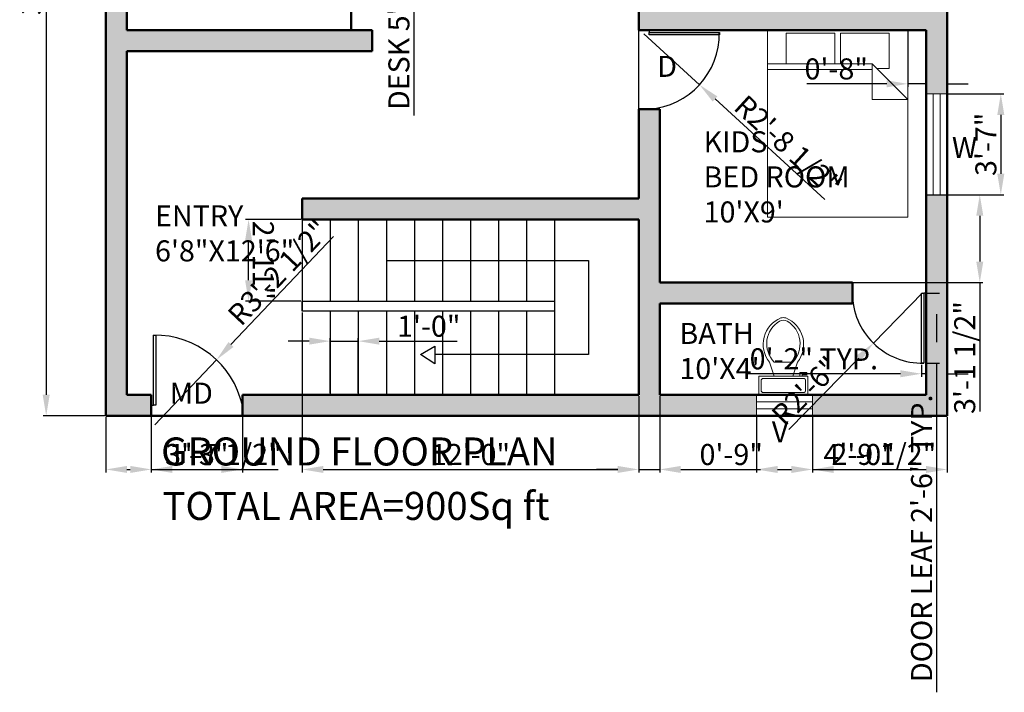
# Model space of a CAD drawing. Units: inches. Extents: x 16989 to 17950, y 7982 to 8536.
# Tile 1 of 5: x 16993 to 17415, y 7982 to 8270. Entities that reach past the tile are written whole.
import ezdxf

# ---------------------------------------------------------------- set-up
doc = ezdxf.new("R2010")
doc.units = ezdxf.units.IN
for name, color, linetype, lineweight in [('A-ANNO-DIMS', 2, 'Continuous', 18), ('A-ANNO-IDEN', 7, 'Continuous', 18), ('A-ANNO-TEXT', 7, 'Continuous', 35), ('A-AREA-IDEN', 7, 'Continuous', 25), ('A-DOOR', 3, 'Continuous', 25), ('A-FLOR-FIXT', 9, 'Continuous', 18), ('A-FLOR-STRS', 7, 'Continuous', 25), ('A-FURN', 8, 'Continuous', 18), ('A-GLAZ', 4, 'Continuous', 18), ('A-WALL', 7, 'Continuous', 50)]:
    doc.layers.add(name, color=color, linetype=linetype, lineweight=lineweight)
doc.layers.add('A-WALL-PATT', color=177, linetype='Continuous', lineweight=13, true_color=0x293189)
doc.styles.get("Standard").update_dxf_attribs({"font": 'arial.ttf'})
doc.dimstyles.new('ISO-25', dxfattribs={"dimtxt": 9, "dimasz": 9, "dimexe": 1.25, "dimexo": 0.625, "dimtad": 1, "dimdec": 1, "dimrnd": 9, "dimlunit": 3, "dimtxsty": 'Standard', "dimcen": 2.5, "dimadec": 0, "dimazin": 0, "dimtfac": 1, "dimtdec": 1, "dimtmove": 0, "dimatfit": 3, "dimfxl": 1, "dimarcsym": 0})

# ---------------------------------------------------------------- blocks, each defined once
blk = doc.blocks.new('Bed - Queen')
for p, q in [((0, -80.00003), (0, 0)), ((0, 0), (59.99999, 0)), ((59.99999, 0), (59.99999, -80.00003)), ((7.99999, -1.2), (28.79998, -1.2)), ((7.99999, -14.4), (7.99999, -1.2)), ((28.79998, -1.2), (28.79998, -14.4)), ((31.19999, -1.2), (51.99999, -1.2)), ((31.19999, -14.4), (31.19999, -1.2)), ((51.99999, -1.2), (51.99999, -16.4)), ((0, -14.4), (44.8, -14.4)), ((44.8, -16.8), (0, -16.8)), ((59.99999, -29.6), (44.8, -14.4)), ((44.8, -14.4), (44.8, -29.6)), ((51.99999, -16.4), (46.79936, -16.4)), ((44.8, -29.6), (59.99999, -29.6)), ((59.99999, -80.00003), (0, -80.00003))]:
    blk.add_line(p, q)
blk = doc.blocks.new('Toilet - top')
for p, q in [((9.5, -6), (9.5, -2)), ((-8, -8.5), (-8, -8)), ((-7, -8), (-7, -9.5)), ((-4, -8), (-6, -14)), ((4, -8), (6, -14)), ((-10, -8.5), (-8, -8.5)), ((-10, -9.5), (-10, -8.5)), ((-7, -9.5), (-10, -9.5)), ((4, -14), (-4, -14))]:
    blk.add_line(p, q)
blk.add_lwpolyline([(10.5, -8), (10.5, 0), (-10.5, 0), (-10.5, -8)], close=True)
for points in [[(-9.5, -2), (-9.5, -6)], [(8.5, -1), (-8.5, -1)], [(-8.5, -7), (8.5, -7)]]:
    blk.add_lwpolyline(points)
for centre, radius, start, end in [((-8.62, -1.88), 0.884, 81.8699, 188.1301), ((8.62, -1.88), 0.884, 351.8699, 98.1301), ((-8.62, -6.12), 0.884, 171.8699, 278.1301), ((8.62, -6.12), 0.884, 261.8699, 8.1301), ((3.52, -21.58), 12.17, 141.4691, 247.9714), ((4.2, -21.82), 11.33, 136.3677, 238.9468), ((-3.52, -21.58), 12.17, 292.0284, 38.5307), ((-4.2, -21.82), 11.33, 301.053, 43.6321), ((0, -27.88), 4, 245.7318, 294.2682), ((0, -29), 4, 254.8605, 285.1395)]:
    blk.add_arc(centre, radius, start, end)
blk = doc.blocks.new('*D9')
at = {"layer": 'A-ANNO-DIMS', "color": 0, "lineweight": -2, "transparency": 16777216}
for p, q in [((17029.59, 8460.26), (17003.42, 8460.26)), ((17004.67, 8451.26), (17004.67, 8109.26)), ((17029.59, 8100.26), (17003.42, 8100.26))]:
    blk.add_line(p, q, dxfattribs=at)
at = {"layer": 'A-ANNO-DIMS', "color": 0, "transparency": 16777216}
for points in [[(17003.17, 8451.26), (17006.17, 8451.26), (17004.67, 8460.26)], [(17003.17, 8109.26), (17006.17, 8109.26), (17004.67, 8100.26)]]:
    blk.add_solid(points, dxfattribs=at)
at = {"layer": 'Defpoints', "color": 0, "transparency": 16777216}
for p in [(17030.22, 8460.26), (17004.67, 8100.26), (17030.22, 8100.26)]:
    blk.add_point(p, dxfattribs=at)
at = {"layer": 'A-ANNO-DIMS', "color": 0, "transparency": 16777216, "insert": (16999.45, 8280.26), "char_height": 9, "attachment_point": 5, "rotation": 90}
blk.add_mtext("30'", dxfattribs=at)
blk = doc.blocks.new('DOOR-LEAF-30IN')
for p, q in [((1, 0), (1, 30)), ((1, 30), (2, 30)), ((2, 30), (2, 0)), ((0, 0), (1, 0)), ((2, 0), (1, 0))]:
    blk.add_line(p, q)
blk = doc.blocks.new('*D17')
at = {"layer": 'A-ANNO-DIMS', "color": 0, "lineweight": -2, "transparency": 16777216}
for p, q in [((17381.84, 8152.76), (17386.97, 8152.76)), ((17385.72, 8143.76), (17385.72, 8131.76)), ((17381.84, 8122.76), (17386.97, 8122.76)), ((17385.72, 8122.76), (17385.72, 7981.95))]:
    blk.add_line(p, q, dxfattribs=at)
at = {"layer": 'A-ANNO-DIMS', "color": 0, "transparency": 16777216}
for points in [[(17384.22, 8143.76), (17387.22, 8143.76), (17385.72, 8152.76)], [(17384.22, 8131.76), (17387.22, 8131.76), (17385.72, 8122.76)]]:
    blk.add_solid(points, dxfattribs=at)
at = {"layer": 'Defpoints', "color": 0, "transparency": 16777216}
for p in [(17381.22, 8152.76), (17381.22, 8122.76), (17385.72, 8122.76)]:
    blk.add_point(p, dxfattribs=at)
at = {"layer": 'A-ANNO-DIMS', "color": 0, "transparency": 16777216, "insert": (17380.44, 8047.85), "char_height": 9, "attachment_point": 5, "rotation": 90}
blk.add_mtext('DOOR LEAF 2\'-6" TYP.', dxfattribs=at)
blk = doc.blocks.new('*D18')
at = {"layer": 'A-ANNO-DIMS', "color": 0, "lineweight": -2, "transparency": 16777216}
for p, q in [((17379.22, 8122.14), (17379.22, 8117.01)), ((17381.22, 8122.14), (17381.22, 8117.01)), ((17370.22, 8118.26), (17305.11, 8118.26)), ((17381.22, 8118.26), (17379.22, 8118.26)), ((17390.22, 8118.26), (17399.22, 8118.26))]:
    blk.add_line(p, q, dxfattribs=at)
at = {"layer": 'A-ANNO-DIMS', "color": 0, "transparency": 16777216}
for points in [[(17370.22, 8119.76), (17370.22, 8116.76), (17379.22, 8118.26)], [(17390.22, 8119.76), (17390.22, 8116.76), (17381.22, 8118.26)]]:
    blk.add_solid(points, dxfattribs=at)
at = {"layer": 'Defpoints', "color": 0, "transparency": 16777216}
for p in [(17379.22, 8122.76), (17381.22, 8122.76), (17379.22, 8118.26)]:
    blk.add_point(p, dxfattribs=at)
at = {"layer": 'A-ANNO-DIMS', "color": 0, "transparency": 16777216, "insert": (17333.16, 8123.48), "char_height": 9, "attachment_point": 5}
blk.add_mtext('0\'-2" TYP.', dxfattribs=at)
blk = doc.blocks.new('*D27')
at = {"layer": 'A-ANNO-DIMS', "color": 0, "lineweight": -2, "transparency": 16777216}
for p, q in [((17170.41, 8391.11), (17160.79, 8391.11)), ((17162.04, 8382.11), (17162.04, 8340.11)), ((17170.41, 8331.11), (17160.79, 8331.11)), ((17162.04, 8331.11), (17162.04, 8228.71))]:
    blk.add_line(p, q, dxfattribs=at)
at = {"layer": 'A-ANNO-DIMS', "color": 0, "transparency": 16777216}
for points in [[(17160.54, 8382.11), (17163.54, 8382.11), (17162.04, 8391.11)], [(17160.54, 8340.11), (17163.54, 8340.11), (17162.04, 8331.11)]]:
    blk.add_solid(points, dxfattribs=at)
at = {"layer": 'Defpoints', "color": 0, "transparency": 16777216}
for p in [(17171.04, 8391.11), (17162.04, 8331.11), (17171.04, 8331.11)]:
    blk.add_point(p, dxfattribs=at)
at = {"layer": 'A-ANNO-DIMS', "color": 0, "transparency": 16777216, "insert": (17156.76, 8275.41), "char_height": 9, "attachment_point": 5, "rotation": 90}
blk.add_mtext('DESK 5\'-0" TYP.', dxfattribs=at)
blk = doc.blocks.new('*D33')
at = {"layer": 'A-ANNO-DIMS', "color": 0, "lineweight": -2, "transparency": 16777216}
for p, q in [((17042.78, 8293.82), (17042.78, 8279.54)), ((17133.78, 8293.82), (17133.78, 8279.54)), ((17051.78, 8280.79), (17124.78, 8280.79)), ((17133.78, 8280.79), (17242.95, 8280.79))]:
    blk.add_line(p, q, dxfattribs=at)
at = {"layer": 'A-ANNO-DIMS', "color": 0, "transparency": 16777216}
for points in [[(17051.78, 8282.29), (17051.78, 8279.29), (17042.78, 8280.79)], [(17124.78, 8282.29), (17124.78, 8279.29), (17133.78, 8280.79)]]:
    blk.add_solid(points, dxfattribs=at)
at = {"layer": 'Defpoints', "color": 0, "transparency": 16777216}
for p in [(17042.78, 8294.44), (17133.78, 8294.44), (17133.78, 8280.79)]:
    blk.add_point(p, dxfattribs=at)
at = {"layer": 'A-ANNO-DIMS', "color": 0, "transparency": 16777216, "insert": (17192.87, 8286.07), "char_height": 9, "attachment_point": 5}
blk.add_mtext('DINING SET 7\'-7"', dxfattribs=at)
blk = doc.blocks.new('*D43')
at = {"layer": 'A-ANNO-DIMS', "color": 0, "lineweight": -2, "transparency": 16777216}
for p, q in [((17381.84, 8194.87), (17405.42, 8194.87)), ((17404.17, 8185.87), (17404.17, 8166.26)), ((17381.84, 8157.26), (17405.42, 8157.26)), ((17404.17, 8157.26), (17404.17, 8102.12))]:
    blk.add_line(p, q, dxfattribs=at)
at = {"layer": 'A-ANNO-DIMS', "color": 0, "transparency": 16777216}
for points in [[(17402.67, 8185.87), (17405.67, 8185.87), (17404.17, 8194.87)], [(17402.67, 8166.26), (17405.67, 8166.26), (17404.17, 8157.26)]]:
    blk.add_solid(points, dxfattribs=at)
at = {"layer": 'Defpoints', "color": 0, "transparency": 16777216}
for p in [(17381.22, 8194.87), (17381.22, 8157.26), (17404.17, 8157.26)]:
    blk.add_point(p, dxfattribs=at)
at = {"layer": 'A-ANNO-DIMS', "color": 0, "transparency": 16777216, "insert": (17398.89, 8125.19), "char_height": 9, "attachment_point": 5, "rotation": 90}
blk.add_mtext('3\'-1 1/2"', dxfattribs=at)
blk = doc.blocks.new('*D44')
at = {"layer": 'A-ANNO-DIMS', "color": 0, "lineweight": -2, "transparency": 16777216}
for p, q in [((17390.84, 8238), (17414.42, 8238)), ((17413.17, 8229), (17413.17, 8203.87)), ((17390.84, 8194.87), (17414.42, 8194.87))]:
    blk.add_line(p, q, dxfattribs=at)
at = {"layer": 'A-ANNO-DIMS', "color": 0, "transparency": 16777216}
for points in [[(17411.67, 8229), (17414.67, 8229), (17413.17, 8238)], [(17411.67, 8203.87), (17414.67, 8203.87), (17413.17, 8194.87)]]:
    blk.add_solid(points, dxfattribs=at)
at = {"layer": 'Defpoints', "color": 0, "transparency": 16777216}
for p in [(17390.22, 8238), (17390.22, 8194.87), (17413.17, 8194.87)]:
    blk.add_point(p, dxfattribs=at)
at = {"layer": 'A-ANNO-DIMS', "color": 0, "transparency": 16777216, "insert": (17407.95, 8216.44), "char_height": 9, "attachment_point": 5, "rotation": 90}
blk.add_mtext('3\'-7"', dxfattribs=at)
blk = doc.blocks.new('*D47')
at = {"layer": 'A-ANNO-DIMS', "color": 0, "lineweight": -2, "transparency": 16777216}
for p, q in [((17030.22, 8099.64), (17030.22, 8076.06)), ((17049.62, 8099.64), (17049.62, 8076.06)), ((17039.22, 8077.31), (17040.62, 8077.31)), ((17049.62, 8077.31), (17103.92, 8077.31))]:
    blk.add_line(p, q, dxfattribs=at)
at = {"layer": 'A-ANNO-DIMS', "color": 0, "transparency": 16777216}
for points in [[(17039.22, 8078.81), (17039.22, 8075.81), (17030.22, 8077.31)], [(17040.62, 8078.81), (17040.62, 8075.81), (17049.62, 8077.31)]]:
    blk.add_solid(points, dxfattribs=at)
at = {"layer": 'Defpoints', "color": 0, "transparency": 16777216}
for p in [(17030.22, 8100.26), (17049.62, 8100.26), (17049.62, 8077.31)]:
    blk.add_point(p, dxfattribs=at)
at = {"layer": 'A-ANNO-DIMS', "color": 0, "transparency": 16777216, "insert": (17081.27, 8082.59), "char_height": 9, "attachment_point": 5}
blk.add_mtext('1\'-7 1/2"', dxfattribs=at)
blk = doc.blocks.new('*D48')
at = {"layer": 'A-ANNO-DIMS', "color": 0, "lineweight": -2, "transparency": 16777216}
for p, q in [((17049.62, 8099.64), (17049.62, 8076.06)), ((17088.6, 8099.64), (17088.6, 8076.06)), ((17058.62, 8077.31), (17079.6, 8077.31))]:
    blk.add_line(p, q, dxfattribs=at)
at = {"layer": 'A-ANNO-DIMS', "color": 0, "transparency": 16777216}
for points in [[(17058.62, 8078.81), (17058.62, 8075.81), (17049.62, 8077.31)], [(17079.6, 8078.81), (17079.6, 8075.81), (17088.6, 8077.31)]]:
    blk.add_solid(points, dxfattribs=at)
at = {"layer": 'Defpoints', "color": 0, "transparency": 16777216}
for p in [(17049.62, 8100.26), (17088.6, 8100.26), (17088.6, 8077.31)]:
    blk.add_point(p, dxfattribs=at)
at = {"layer": 'A-ANNO-DIMS', "color": 0, "transparency": 16777216, "insert": (17069.11, 8082.53), "char_height": 9, "attachment_point": 5}
blk.add_mtext('3\'-3"', dxfattribs=at)
blk = doc.blocks.new('*D49')
at = {"layer": 'A-ANNO-DIMS', "color": 0, "lineweight": -2, "transparency": 16777216}
for p, q in [((17308.63, 8099.64), (17308.63, 8076.06)), ((17332.58, 8099.64), (17332.58, 8076.06)), ((17317.63, 8077.31), (17323.58, 8077.31)), ((17332.58, 8077.31), (17366.91, 8077.31))]:
    blk.add_line(p, q, dxfattribs=at)
at = {"layer": 'A-ANNO-DIMS', "color": 0, "transparency": 16777216}
for points in [[(17317.63, 8078.81), (17317.63, 8075.81), (17308.63, 8077.31)], [(17323.58, 8078.81), (17323.58, 8075.81), (17332.58, 8077.31)]]:
    blk.add_solid(points, dxfattribs=at)
at = {"layer": 'Defpoints', "color": 0, "transparency": 16777216}
for p in [(17308.63, 8100.26), (17332.58, 8100.26), (17332.58, 8077.31)]:
    blk.add_point(p, dxfattribs=at)
at = {"layer": 'A-ANNO-DIMS', "color": 0, "transparency": 16777216, "insert": (17354.25, 8082.53), "char_height": 9, "attachment_point": 5}
blk.add_mtext('2\'-0"', dxfattribs=at)
blk = doc.blocks.new('*D50')
at = {"layer": 'A-ANNO-DIMS', "color": 0, "lineweight": -2, "transparency": 16777216}
for p, q in [((17332.58, 8099.64), (17332.58, 8076.06)), ((17390.22, 8099.64), (17390.22, 8076.06)), ((17341.58, 8077.31), (17381.22, 8077.31))]:
    blk.add_line(p, q, dxfattribs=at)
at = {"layer": 'A-ANNO-DIMS', "color": 0, "transparency": 16777216}
for points in [[(17341.58, 8078.81), (17341.58, 8075.81), (17332.58, 8077.31)], [(17381.22, 8078.81), (17381.22, 8075.81), (17390.22, 8077.31)]]:
    blk.add_solid(points, dxfattribs=at)
at = {"layer": 'Defpoints', "color": 0, "transparency": 16777216}
for p in [(17332.58, 8100.26), (17390.22, 8100.26), (17390.22, 8077.31)]:
    blk.add_point(p, dxfattribs=at)
at = {"layer": 'A-ANNO-DIMS', "color": 0, "transparency": 16777216, "insert": (17361.4, 8082.59), "char_height": 9, "attachment_point": 5}
blk.add_mtext('4\'-9 1/2"', dxfattribs=at)
blk = doc.blocks.new('*D61')
at = {"layer": 'A-ANNO-DIMS', "color": 0, "lineweight": -2, "transparency": 16777216}
for p, q in [((17114.22, 8144.4), (17114.22, 8076.06)), ((17258.22, 8108.64), (17258.22, 8076.06)), ((17123.22, 8077.31), (17249.22, 8077.31))]:
    blk.add_line(p, q, dxfattribs=at)
at = {"layer": 'A-ANNO-DIMS', "color": 0, "transparency": 16777216}
for points in [[(17123.22, 8078.81), (17123.22, 8075.81), (17114.22, 8077.31)], [(17249.22, 8078.81), (17249.22, 8075.81), (17258.22, 8077.31)]]:
    blk.add_solid(points, dxfattribs=at)
at = {"layer": 'Defpoints', "color": 0, "transparency": 16777216}
for p in [(17114.22, 8145.02), (17258.22, 8109.26), (17258.22, 8077.31)]:
    blk.add_point(p, dxfattribs=at)
at = {"layer": 'A-ANNO-DIMS', "color": 0, "transparency": 16777216, "insert": (17186.22, 8082.53), "char_height": 9, "attachment_point": 5}
blk.add_mtext('12\'-0"', dxfattribs=at)
blk = doc.blocks.new('*D62')
at = {"layer": 'A-ANNO-DIMS', "color": 0, "lineweight": -2, "transparency": 16777216}
for p, q in [((17113.59, 8184.26), (17090.01, 8184.25)), ((17091.27, 8158.3), (17091.26, 8175.25)), ((17113.59, 8149.31), (17090.02, 8149.3))]:
    blk.add_line(p, q, dxfattribs=at)
at = {"layer": 'A-ANNO-DIMS', "color": 0, "transparency": 16777216}
for points in [[(17092.76, 8175.26), (17089.76, 8175.25), (17091.26, 8184.25)], [(17092.77, 8158.3), (17089.77, 8158.3), (17091.27, 8149.3)]]:
    blk.add_solid(points, dxfattribs=at)
at = {"layer": 'Defpoints', "color": 0, "transparency": 16777216}
for p in [(17091.26, 8184.25), (17114.21, 8184.26), (17114.22, 8149.31)]:
    blk.add_point(p, dxfattribs=at)
at = {"layer": 'A-ANNO-DIMS', "color": 0, "transparency": 16777216, "insert": (17096.41, 8166.78), "char_height": 9, "attachment_point": 5, "rotation": 270.0146}
blk.add_mtext('2\'-11"', dxfattribs=at)
blk = doc.blocks.new('*D63')
at = {"layer": 'A-ANNO-DIMS', "color": 0, "lineweight": -2, "transparency": 16777216}
for p, q in [((17117.22, 8132.21), (17108.22, 8132.21)), ((17126.22, 8109.89), (17126.22, 8133.46)), ((17126.22, 8132.21), (17138.22, 8132.21)), ((17138.22, 8109.89), (17138.22, 8133.46)), ((17147.22, 8132.21), (17180.55, 8132.21))]:
    blk.add_line(p, q, dxfattribs=at)
at = {"layer": 'A-ANNO-DIMS', "color": 0, "transparency": 16777216}
for points in [[(17117.22, 8133.71), (17117.22, 8130.71), (17126.22, 8132.21)], [(17147.22, 8133.71), (17147.22, 8130.71), (17138.22, 8132.21)]]:
    blk.add_solid(points, dxfattribs=at)
at = {"layer": 'Defpoints', "color": 0, "transparency": 16777216}
for p in [(17138.22, 8132.21), (17126.22, 8109.26), (17138.22, 8109.26)]:
    blk.add_point(p, dxfattribs=at)
at = {"layer": 'A-ANNO-DIMS', "color": 0, "transparency": 16777216, "insert": (17168.38, 8137.43), "char_height": 9, "attachment_point": 5}
blk.add_mtext('1\'-0"', dxfattribs=at)
blk = doc.blocks.new('*D67')
at = {"layer": 'A-ANNO-DIMS', "color": 0, "lineweight": -2, "transparency": 16777216}
for p, q in [((17258.22, 8108.64), (17258.22, 8076.06)), ((17267.22, 8108.64), (17267.22, 8076.06)), ((17249.22, 8077.31), (17240.22, 8077.31)), ((17258.22, 8077.31), (17267.22, 8077.31)), ((17276.22, 8077.31), (17310.39, 8077.31))]:
    blk.add_line(p, q, dxfattribs=at)
at = {"layer": 'A-ANNO-DIMS', "color": 0, "transparency": 16777216}
for points in [[(17249.22, 8078.81), (17249.22, 8075.81), (17258.22, 8077.31)], [(17276.22, 8078.81), (17276.22, 8075.81), (17267.22, 8077.31)]]:
    blk.add_solid(points, dxfattribs=at)
at = {"layer": 'Defpoints', "color": 0, "transparency": 16777216}
for p in [(17258.22, 8109.26), (17267.22, 8109.26), (17267.22, 8077.31)]:
    blk.add_point(p, dxfattribs=at)
at = {"layer": 'A-ANNO-DIMS', "color": 0, "transparency": 16777216, "insert": (17297.81, 8082.53), "char_height": 9, "attachment_point": 5}
blk.add_mtext('0\'-9"', dxfattribs=at)
blk = doc.blocks.new('*D69')
at = {"layer": 'A-ANNO-DIMS', "color": 0, "lineweight": -2, "transparency": 16777216}
for p, q in [((17373.35, 8264.64), (17373.35, 8241.06)), ((17381.22, 8264.64), (17381.22, 8241.06)), ((17364.35, 8242.31), (17330.18, 8242.31)), ((17381.22, 8242.31), (17373.35, 8242.31)), ((17390.22, 8242.31), (17399.22, 8242.31))]:
    blk.add_line(p, q, dxfattribs=at)
at = {"layer": 'A-ANNO-DIMS', "color": 0, "transparency": 16777216}
for points in [[(17364.35, 8243.81), (17364.35, 8240.81), (17373.35, 8242.31)], [(17390.22, 8243.81), (17390.22, 8240.81), (17381.22, 8242.31)]]:
    blk.add_solid(points, dxfattribs=at)
at = {"layer": 'Defpoints', "color": 0, "transparency": 16777216}
for p in [(17373.35, 8265.26), (17381.22, 8265.26), (17373.35, 8242.31)]:
    blk.add_point(p, dxfattribs=at)
at = {"layer": 'A-ANNO-DIMS', "color": 0, "transparency": 16777216, "insert": (17342.76, 8247.53), "char_height": 9, "attachment_point": 5}
blk.add_mtext('0\'-8"', dxfattribs=at)
blk = doc.blocks.new('*D72')
at = {"layer": 'A-ANNO-DIMS', "color": 0, "lineweight": -2, "transparency": 16777216}
for p, q in [((17260.37, 8263.76), (17284.23, 8241.92)), ((17337.9, 8192.78), (17290.87, 8235.84))]:
    blk.add_line(p, q, dxfattribs=at)
at = {"layer": 'A-ANNO-DIMS', "color": 0, "transparency": 16777216}
blk.add_solid([(17291.88, 8236.94), (17289.86, 8234.73), (17284.23, 8241.92)], dxfattribs=at)
at = {"layer": 'Defpoints', "color": 0, "transparency": 16777216}
for p in [(17260.37, 8263.76), (17284.23, 8241.92)]:
    blk.add_point(p, dxfattribs=at)
at = {"layer": 'A-ANNO-DIMS', "color": 0, "transparency": 16777216, "insert": (17321.27, 8215.16), "char_height": 9, "attachment_point": 5, "rotation": 317.522}
blk.add_mtext('R2\'-8 1/2"', dxfattribs=at)
blk = doc.blocks.new('*D74')
at = {"layer": 'A-ANNO-DIMS', "color": 0, "lineweight": -2, "transparency": 16777216}
for p, q in [((17379.72, 8152.84), (17358.65, 8131.36)), ((17322.39, 8094.39), (17352.35, 8124.94))]:
    blk.add_line(p, q, dxfattribs=at)
at = {"layer": 'A-ANNO-DIMS', "color": 0, "transparency": 16777216}
blk.add_solid([(17351.28, 8125.99), (17353.42, 8123.89), (17358.65, 8131.36)], dxfattribs=at)
at = {"layer": 'Defpoints', "color": 0, "transparency": 16777216}
for p in [(17379.72, 8152.84), (17358.65, 8131.36)]:
    blk.add_point(p, dxfattribs=at)
at = {"layer": 'A-ANNO-DIMS', "color": 0, "transparency": 16777216, "insert": (17330.49, 8110.11), "char_height": 9, "attachment_point": 5, "rotation": 45.552}
blk.add_mtext('R2\'-6"', dxfattribs=at)
blk = doc.blocks.new('*D76')
at = {"layer": 'A-ANNO-DIMS', "color": 0, "lineweight": -2, "transparency": 16777216}
for p, q in [((17127.6, 8177.04), (17083.74, 8130.76)), ((17051.12, 8096.36), (17077.55, 8124.23))]:
    blk.add_line(p, q, dxfattribs=at)
at = {"layer": 'A-ANNO-DIMS', "color": 0, "transparency": 16777216}
blk.add_solid([(17082.65, 8131.8), (17084.83, 8129.73), (17077.55, 8124.23)], dxfattribs=at)
at = {"layer": 'Defpoints', "color": 0, "transparency": 16777216}
for p in [(17077.55, 8124.23), (17051.12, 8096.36)]:
    blk.add_point(p, dxfattribs=at)
at = {"layer": 'A-ANNO-DIMS', "color": 0, "transparency": 16777216, "insert": (17104.93, 8160.8), "char_height": 9, "attachment_point": 5, "rotation": 46.5334}
blk.add_mtext('R3\'-2 1/2"', dxfattribs=at)

msp = doc.modelspace()

# ---------------------------------------------------------------- hatches: boundary and pattern name
at = {"layer": 'A-WALL-PATT'}
h = msp.add_hatch(color=256, dxfattribs=at)
h.dxf.hatch_style = 1
h.paths.add_polyline_path([(17039.22, 8310.16), (17030.22, 8310.16), (17030.22, 8100.26), (17049.62, 8100.26), (17049.62, 8109.26), (17039.22, 8109.26), (17039.22, 8256.26), (17144.22, 8256.26), (17144.22, 8265.26), (17039.22, 8265.26)])
h.paths.add_polyline_path([(17039.22, 8451.26), (17065.89, 8451.26), (17065.89, 8460.26), (17030.22, 8460.26), (17030.22, 8357.88), (17039.22, 8357.88)])
h.paths.add_polyline_path([(17180.39, 8460.26), (17105.01, 8460.26), (17105.01, 8451.26), (17135.22, 8451.26), (17135.22, 8333.76), (17144.22, 8333.76), (17144.22, 8451.26), (17180.39, 8451.26)])
h.paths.add_polyline_path([(17309.67, 8460.26), (17217.66, 8460.26), (17217.66, 8451.26), (17258.22, 8451.26), (17258.22, 8304.98), (17262.72, 8304.98, -0.013209), (17264.26, 8304.98), (17267.22, 8304.98), (17267.22, 8394.26), (17348.26, 8394.26), (17348.26, 8403.26), (17267.22, 8403.26), (17267.22, 8451.26), (17309.67, 8451.26)])
h.paths.add_polyline_path([(17390.22, 8460.26), (17336.17, 8460.26), (17336.17, 8451.26), (17381.22, 8451.26), (17381.22, 8403.26), (17381.22, 8394.26), (17381.22, 8367.17), (17390.22, 8367.17)])
h.paths.add_polyline_path([(17390.22, 8325.05), (17381.22, 8325.05), (17381.22, 8274.26), (17267.22, 8274.26), (17258.22, 8274.26), (17258.22, 8265.26), (17267.22, 8265.26), (17381.22, 8265.26), (17381.22, 8238), (17390.22, 8238)])
h.paths.add_polyline_path([(17390.22, 8194.87), (17381.22, 8194.87), (17381.22, 8157.26), (17381.22, 8148.26), (17381.22, 8109.26), (17332.58, 8109.26), (17332.58, 8100.26), (17390.22, 8100.26)])
h.paths.add_polyline_path([(17349.64, 8157.26), (17267.22, 8157.26), (17267.22, 8231.5), (17258.22, 8231.5), (17258.22, 8193.26), (17144.22, 8193.26), (17114.21, 8193.26), (17114.21, 8184.26), (17144.22, 8184.26), (17258.22, 8184.26), (17258.22, 8109.26), (17088.6, 8109.26), (17088.6, 8100.26), (17308.63, 8100.26), (17308.63, 8109.26), (17267.22, 8109.26), (17267.22, 8148.26), (17349.64, 8148.26)])

# ---------------------------------------------------------------- linework, layer by layer
at = {"layer": 'A-DOOR'}
for p, q in [((17258.22, 8231.5), (17258.22, 8265.26)), ((17349.64, 8157.26), (17381.22, 8157.26))]:
    msp.add_line(p, q, dxfattribs=at)
for centre, radius, start, end in [((17260.37, 8263.76), 32.35, 274.1572, 0.8856), ((17379.72, 8152.84), 30.08, 180.1517, 270.9523), ((17051.12, 8096.36), 38.41, 12.64, 90.7459)]:
    msp.add_arc(centre, radius, start, end, dxfattribs=at)
at = {"layer": 'A-FLOR-STRS'}
for p, q in [((17114.22, 8184.26), (17114.22, 8145.02)), ((17126.22, 8184.26), (17126.22, 8149.31)), ((17138.22, 8184.26), (17138.22, 8149.31)), ((17150.22, 8184.26), (17150.22, 8149.31)), ((17162.22, 8184.26), (17162.22, 8149.31)), ((17174.22, 8184.26), (17174.22, 8149.31)), ((17186.22, 8184.26), (17186.22, 8149.31)), ((17198.22, 8184.26), (17198.22, 8149.31)), ((17210.22, 8184.26), (17210.22, 8149.31)), ((17222.22, 8184.26), (17222.22, 8109.26)), ((17150.22, 8166.79), (17236.68, 8166.79)), ((17236.68, 8166.79), (17236.68, 8126.43)), ((17126.22, 8145.02), (17126.22, 8109.26)), ((17138.22, 8145.02), (17138.22, 8109.26)), ((17150.22, 8145.02), (17150.22, 8109.26)), ((17162.22, 8145.02), (17162.22, 8109.26)), ((17174.22, 8145.02), (17174.22, 8109.26)), ((17186.22, 8145.02), (17186.22, 8109.26)), ((17198.22, 8145.02), (17198.22, 8109.26)), ((17210.22, 8145.02), (17210.22, 8109.26)), ((17164.87, 8126.43), (17171.03, 8130.06)), ((17171.03, 8130.06), (17171.03, 8122.45)), ((17171.03, 8122.45), (17164.87, 8126.43)), ((17236.68, 8126.43), (17171.03, 8126.43))]:
    msp.add_line(p, q, dxfattribs=at)
msp.add_lwpolyline([(17222.22, 8145.02), (17114.22, 8145.02), (17114.22, 8149.31), (17222.22, 8149.31)], close=True, dxfattribs=at)
at = {"layer": 'A-GLAZ'}
for p, q in [((17381.22, 8238), (17390.22, 8238)), ((17384.22, 8194.87), (17384.22, 8238)), ((17387.22, 8194.87), (17387.22, 8238)), ((17381.22, 8194.87), (17390.22, 8194.87)), ((17308.63, 8109.26), (17308.63, 8100.26)), ((17332.58, 8109.26), (17332.58, 8100.26)), ((17308.63, 8106.26), (17332.58, 8106.26)), ((17308.63, 8103.26), (17332.58, 8103.26))]:
    msp.add_line(p, q, dxfattribs=at)
at = {"layer": 'A-WALL'}
for p, q in [((17030.22, 8460.26), (17030.22, 8100.26)), ((17390.22, 8100.26), (17390.22, 8460.26)), ((17039.22, 8451.26), (17039.22, 8265.26)), ((17135.22, 8451.26), (17135.22, 8265.26)), ((17258.22, 8274.26), (17258.22, 8265.26)), ((17144.22, 8265.26), (17039.22, 8265.26)), ((17144.22, 8265.26), (17144.22, 8256.26)), ((17267.22, 8265.26), (17258.22, 8265.26)), ((17381.22, 8265.26), (17267.22, 8265.26)), ((17381.22, 8157.26), (17381.22, 8265.26)), ((17144.22, 8256.26), (17039.22, 8256.26)), ((17039.22, 8256.26), (17039.22, 8109.26)), ((17267.22, 8231.5), (17258.22, 8231.5)), ((17258.22, 8231.5), (17258.22, 8193.26)), ((17267.22, 8231.5), (17267.22, 8157.26)), ((17144.22, 8193.26), (17114.21, 8193.26)), ((17114.21, 8193.26), (17114.21, 8184.26)), ((17258.22, 8193.26), (17144.22, 8193.26)), ((17114.21, 8184.26), (17144.22, 8184.26)), ((17258.22, 8184.26), (17144.22, 8184.26)), ((17258.22, 8184.26), (17258.22, 8109.26)), ((17349.64, 8157.26), (17267.22, 8157.26)), ((17349.64, 8157.26), (17349.64, 8148.26)), ((17381.22, 8157.26), (17381.22, 8148.26)), ((17349.64, 8148.26), (17267.22, 8148.26)), ((17267.22, 8148.26), (17267.22, 8109.26)), ((17381.22, 8109.26), (17381.22, 8148.26)), ((17039.22, 8109.26), (17049.62, 8109.26)), ((17049.62, 8109.26), (17049.62, 8100.26)), ((17088.6, 8109.26), (17258.22, 8109.26)), ((17088.6, 8109.26), (17088.6, 8100.26)), ((17267.22, 8109.26), (17381.22, 8109.26)), ((17030.22, 8100.26), (17390.22, 8100.26))]:
    msp.add_line(p, q, dxfattribs=at)

# ---------------------------------------------------------------- block references
at = {"layer": 'A-DOOR'}
for p, rotation in [((17262.72, 8265.26), 269.9999999999999), ((17381.22, 8152.76), 180)]:
    msp.add_blockref('DOOR-LEAF-30IN', p, dxfattribs=dict(at, rotation=rotation))
msp.add_blockref('DOOR-LEAF-30IN', (17049.62, 8104.76), dxfattribs=at)
at = {"layer": 'A-FLOR-FIXT', "rotation": 180}
msp.add_blockref('Toilet - top', (17320.14, 8109.26), dxfattribs=at)
at = {"layer": 'A-FURN'}
msp.add_blockref('Bed - Queen', (17313.35, 8265.26), dxfattribs=at)

# ---------------------------------------------------------------- texts
at = {"layer": 'A-ANNO-IDEN', "char_height": 9, "attachment_point": 1}
for s, insert in [('D', (17266.15, 8254.29)), ('W', (17392.26, 8219.52)), ('MD', (17057.56, 8114.44)), ('V', (17315.19, 8097.85))]:
    msp.add_mtext_dynamic_manual_height_columns(s, width=19.3379, gutter_width=12.5, heights=[0], dxfattribs=dict(at, insert=insert))
at = {"layer": 'A-ANNO-TEXT', "char_height": 12, "attachment_point": 1}
for s, insert in [('GROUND FLOOR PLAN', (17053.83, 8091)), ('TOTAL AREA=900Sq ft', (17054.45, 8067.7))]:
    msp.add_mtext_dynamic_manual_height_columns(s, width=318.491, gutter_width=12.5, heights=[0], dxfattribs=dict(at, insert=insert))
at = {"layer": 'A-AREA-IDEN', "char_height": 9, "attachment_point": 1}
for s, width, insert in [("KIDS\\PBED ROOM\\P10'X9'", 99.1602, (17285.99, 8222)), ('ENTRY\\P6\'8"X12\'6"', 65.8099, (17051.24, 8190.34)), ("BATH\\P10'X4'", 65.8099, (17275.63, 8139.99))]:
    msp.add_mtext_dynamic_manual_height_columns(s, width=width, gutter_width=12.5, heights=[0], dxfattribs=dict(at, insert=insert))

# ---------------------------------------------------------------- dimensions: what is measured, and where the dimension line sits
at = {"layer": 'A-ANNO-DIMS'}
for base, p1, p2, angle, override, picture, middle in [((17004.67, 8100.26), (17030.22, 8460.26), (17030.22, 8100.26), 90, {"dimclrd": 0, "dimclre": 0, "dimclrt": 0}, '*D9', (16999.45, 8280.26)), ((17373.35, 8242.31), (17381.22, 8265.26), (17373.35, 8265.26), 180, {"dimdec": 1, "dimlfac": 1, "dimrnd": 0, "dimzin": 1, "dimdsep": 46, "dimlunit": 4, "dimfrac": 2}, '*D69', (17342.76, 8247.53)), ((17413.17, 8194.87), (17390.22, 8238), (17390.22, 8194.87), 90, {"dimdec": 1, "dimlfac": 1, "dimrnd": 0, "dimzin": 1, "dimdsep": 46, "dimlunit": 4, "dimfrac": 2}, '*D44', (17407.95, 8216.44)), ((17404.17, 8157.26), (17381.22, 8194.87), (17381.22, 8157.26), 270, {"dimdec": 1, "dimlfac": 1, "dimrnd": 0, "dimzin": 1, "dimdsep": 46, "dimlunit": 4, "dimfrac": 2}, '*D43', (17398.89, 8125.19)), ((17091.26, 8184.25), (17114.22, 8149.31), (17114.21, 8184.26), 90.0146, {"dimdec": 1, "dimlfac": 1, "dimrnd": 0, "dimzin": 1, "dimdsep": 46, "dimlunit": 4, "dimfrac": 2}, '*D62', (17096.41, 8166.78))]:
    dim = msp.add_linear_dim(base=base, p1=p1, p2=p2, angle=angle, dimstyle='ISO-25', override=override, dxfattribs=at)
    dim.commit()
    dim.dimension.update_dxf_attribs({"geometry": picture, "text_midpoint": middle})
for base, p1, p2, angle, text, picture, middle in [((17162.04, 8331.11), (17171.04, 8391.11), (17171.04, 8331.11), 270, 'DESK <> TYP.', '*D27', (17156.76, 8275.41)), ((17385.72, 8122.76), (17381.22, 8152.76), (17381.22, 8122.76), 270, 'DOOR LEAF <> TYP.', '*D17', (17380.44, 8047.85)), ((17379.22, 8118.26), (17381.22, 8122.76), (17379.22, 8122.76), 180, '<> TYP.', '*D18', (17333.16, 8123.48))]:
    dim = msp.add_linear_dim(base=base, p1=p1, p2=p2, angle=angle, text=text, dimstyle='ISO-25', override={"dimdec": 1, "dimlfac": 1, "dimrnd": 0, "dimzin": 1, "dimdsep": 46, "dimlunit": 4, "dimfrac": 2}, dxfattribs=at)
    dim.commit()
    dim.dimension.update_dxf_attribs({"geometry": picture, "text_midpoint": middle})
dim = msp.add_linear_dim(base=(17133.78, 8280.79), p1=(17042.78, 8294.44), p2=(17133.78, 8294.44), text='DINING SET <>', dimstyle='ISO-25', override={"dimdec": 1, "dimlfac": 1, "dimrnd": 0, "dimzin": 1, "dimdsep": 46, "dimlunit": 4, "dimfrac": 2}, dxfattribs=at)
dim.commit()
dim.dimension.update_dxf_attribs({"geometry": '*D33', "text_midpoint": (17192.87, 8286.07)})
for center, mpoint, picture, middle in [((17260.37, 8263.76), (17284.23, 8241.92), '*D72', (17321.27, 8215.16)), ((17051.12, 8096.36), (17077.55, 8124.23), '*D76', (17104.93, 8160.8)), ((17379.72, 8152.84), (17358.65, 8131.36), '*D74', (17330.49, 8110.11))]:
    dim = msp.add_radius_dim(center=center, mpoint=mpoint, dimstyle='ISO-25', override={"dimdec": 1, "dimlfac": 1, "dimrnd": 0, "dimzin": 1, "dimdsep": 46, "dimlunit": 4, "dimfrac": 2}, dxfattribs=at)
    dim.commit()
    dim.dimension.update_dxf_attribs({"geometry": picture, "text_midpoint": middle})
for base, p1, p2, picture, middle in [((17258.22, 8077.31), (17114.22, 8145.02), (17258.22, 8109.26), '*D61', (17186.22, 8082.53)), ((17138.22, 8132.21), (17126.22, 8109.26), (17138.22, 8109.26), '*D63', (17168.38, 8137.43)), ((17267.22, 8077.31), (17258.22, 8109.26), (17267.22, 8109.26), '*D67', (17297.81, 8082.53)), ((17049.62, 8077.31), (17030.22, 8100.26), (17049.62, 8100.26), '*D47', (17081.27, 8082.59)), ((17088.6, 8077.31), (17049.62, 8100.26), (17088.6, 8100.26), '*D48', (17069.11, 8082.53)), ((17332.5847, 8077.3106), (17308.6312, 8100.2606), (17332.5847, 8100.2606), '*D49', (17354.2486, 8082.5308)), ((17390.22, 8077.31), (17332.58, 8100.26), (17390.22, 8100.26), '*D50', (17361.4, 8082.59))]:
    dim = msp.add_linear_dim(base=base, p1=p1, p2=p2, dimstyle='ISO-25', override={"dimdec": 1, "dimlfac": 1, "dimrnd": 0, "dimzin": 1, "dimdsep": 46, "dimlunit": 4, "dimfrac": 2}, dxfattribs=at)
    dim.commit()
    dim.dimension.update_dxf_attribs({"geometry": picture, "text_midpoint": middle})

doc.saveas('drawing.dxf')
